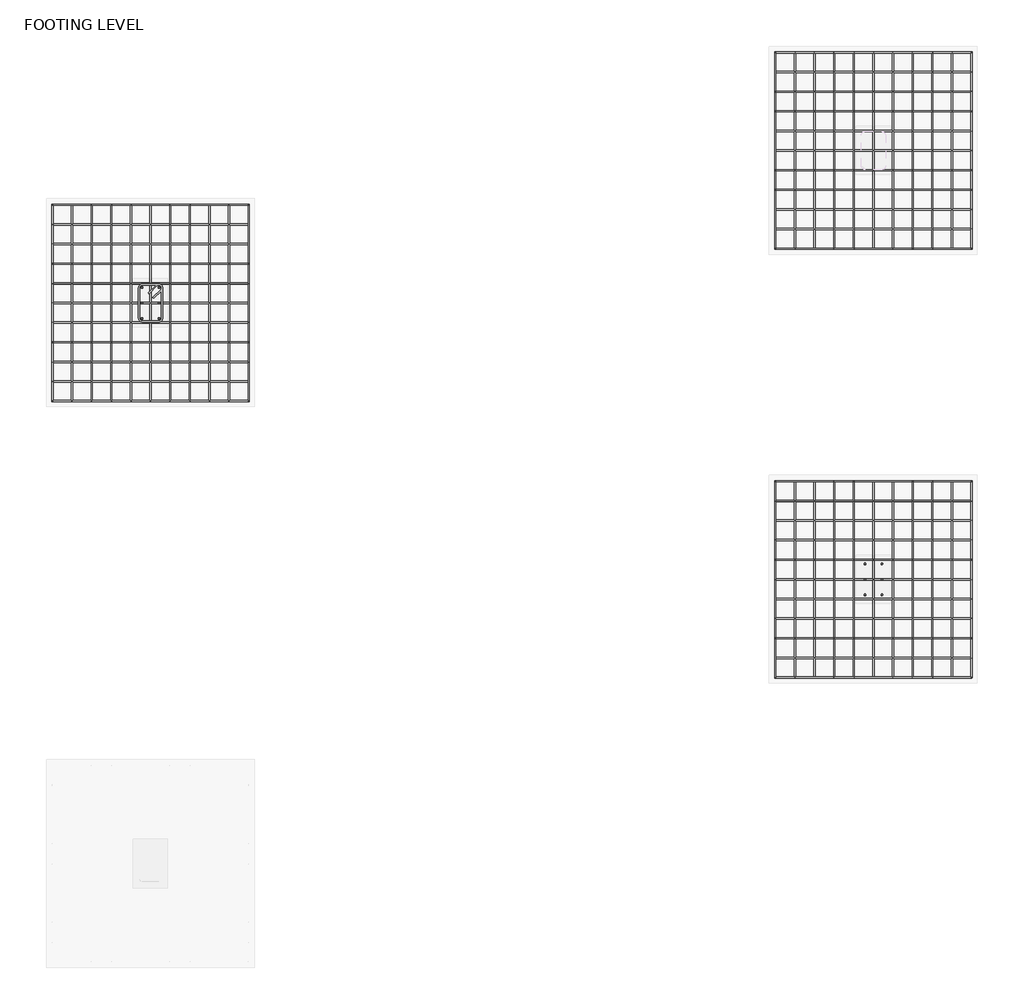
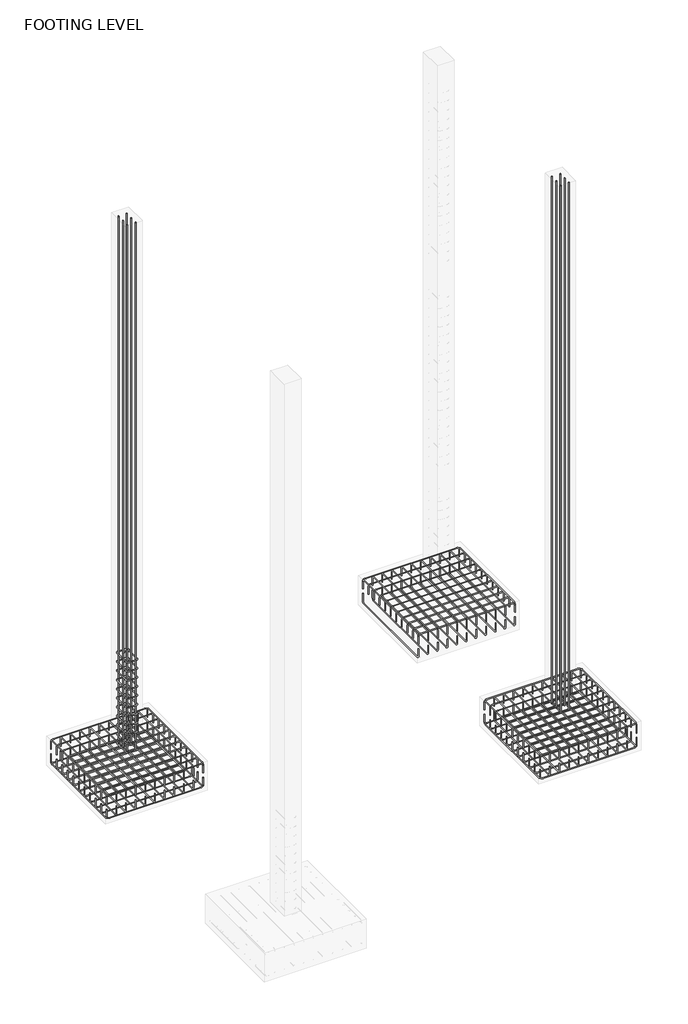
# One storey, part 5 of 9: 24 reinforcing bars.
"""IFC4 building model written with IfcOpenShell, lengths in millimetres."""

from ifc_helpers import new_model, si_unit, point, frame, origin, place, context, project, spatial, polyline, circle_curve, trimmed, segment, composite_curve, source, transform, mapped, element, save
from ifc_brep_helpers import swept_disk

model = new_model("IFC4")

# Units and contexts
model_context = context("Model", 3, world=origin())
ifc_project = project(units=[si_unit("LENGTHUNIT", "METRE", prefix="MILLI")], contexts=[model_context])

# Site, building, storey
site = spatial("IfcSite", under=ifc_project)
building = spatial("IfcBuilding", under=site)
storey = spatial("IfcBuildingStorey", under=building, Name="FOOTING LEVEL", Elevation=-1981.2)

# Reinforcing bars
placement = place(None, origin())
reinforcing_bar_shape = source(origin(), model_context, "Body", "SolidModel", [
    swept_disk(composite_curve([segment(polyline([(-2537.1816189, 2241.6973175, -2171.7), (-2537.1816189, 2241.6973175, -2057.4)]), True, "CONTINUOUS"), segment(trimmed(circle_curve(frame((-2537.1816189, 2208.3598175, -2057.4), z_axis=(1.0, 0.0, 0.0), x_axis=(0.0, 33.337499999999636, 0.0)), 33.3375), [point((-2537.1816189, 2241.6973175, -2057.4))], [point((-2537.1816189, 2208.3598175, -2024.0625))], True, "CARTESIAN"), True, "CONTINUOUS"), segment(polyline([(-2537.1816189, 2208.3598175, -2024.0625), (-2537.1816189, 836.7598175, -2024.0625)]), True, "CONTINUOUS"), segment(trimmed(circle_curve(frame((-2537.1816189, 836.7598175, -2057.4), z_axis=(1.0, 0.0, 0.0), x_axis=(0.0, 0.0, 33.33750000000009)), 33.3375), [point((-2537.1816189, 836.7598175, -2024.0625))], [point((-2537.1816189, 803.4223175, -2057.4))], True, "CARTESIAN"), True, "CONTINUOUS"), segment(polyline([(-2537.1816189, 803.4223175, -2057.4), (-2537.1816189, 803.4223175, -2171.7)]), True, "CONTINUOUS")], self_intersect=False), 4.7625),
])
element("IfcReinforcingBar", 1, at=placement, inside=storey, context=model_context, shape_type="MappedRepresentation", body=[
    mapped(reinforcing_bar_shape, transform((0.0, 0.0, 0.0), x_axis=(1.0, 0.0, 0.0), y_axis=(0.0, 1.0, 0.0), z_axis=(0.0, 0.0, 1.0))),
    mapped(reinforcing_bar_shape, transform((-143.8275, 0.0, 0.0), x_axis=(1.0, 0.0, 0.0), y_axis=(0.0, 1.0, 0.0), z_axis=(0.0, 0.0, 1.0))),
    mapped(reinforcing_bar_shape, transform((-287.655, 0.0, 0.0), x_axis=(1.0, 0.0, 0.0), y_axis=(0.0, 1.0, 0.0), z_axis=(0.0, 0.0, 1.0))),
    mapped(reinforcing_bar_shape, transform((-431.4825, 0.0, 0.0), x_axis=(1.0, 0.0, 0.0), y_axis=(0.0, 1.0, 0.0), z_axis=(0.0, 0.0, 1.0))),
    mapped(reinforcing_bar_shape, transform((-575.31, 0.0, 0.0), x_axis=(1.0, 0.0, 0.0), y_axis=(0.0, 1.0, 0.0), z_axis=(0.0, 0.0, 1.0))),
    mapped(reinforcing_bar_shape, transform((-719.1375, 0.0, 0.0), x_axis=(1.0, 0.0, 0.0), y_axis=(0.0, 1.0, 0.0), z_axis=(0.0, 0.0, 1.0))),
    mapped(reinforcing_bar_shape, transform((-862.965, 0.0, 0.0), x_axis=(1.0, 0.0, 0.0), y_axis=(0.0, 1.0, 0.0), z_axis=(0.0, 0.0, 1.0))),
    mapped(reinforcing_bar_shape, transform((-1006.7925, 0.0, 0.0), x_axis=(1.0, 0.0, 0.0), y_axis=(0.0, 1.0, 0.0), z_axis=(0.0, 0.0, 1.0))),
    mapped(reinforcing_bar_shape, transform((-1150.62, 0.0, 0.0), x_axis=(1.0, 0.0, 0.0), y_axis=(0.0, 1.0, 0.0), z_axis=(0.0, 0.0, 1.0))),
    mapped(reinforcing_bar_shape, transform((-1294.4475, 0.0, 0.0), x_axis=(1.0, 0.0, 0.0), y_axis=(0.0, 1.0, 0.0), z_axis=(0.0, 0.0, 1.0))),
    mapped(reinforcing_bar_shape, transform((-1438.275, 0.0, 0.0), x_axis=(1.0, 0.0, 0.0), y_axis=(0.0, 1.0, 0.0), z_axis=(0.0, 0.0, 1.0))),
])
reinforcing_bar_2_shape = source(origin(), model_context, "Body", "SolidModel", [
    swept_disk(composite_curve([segment(polyline([(-2537.1816189, 803.4223175, -2247.9), (-2537.1816189, 803.4223175, -2362.2)]), True, "CONTINUOUS"), segment(trimmed(circle_curve(frame((-2537.1816189, 836.7598175, -2362.2), z_axis=(1.0, 0.0, 0.0), x_axis=(0.0, -33.33750000000009, 0.0)), 33.3375), [point((-2537.1816189, 803.4223175, -2362.2))], [point((-2537.1816189, 836.7598175, -2395.5375))], True, "CARTESIAN"), True, "CONTINUOUS"), segment(polyline([(-2537.1816189, 836.7598175, -2395.5375), (-2537.1816189, 2208.3598175, -2395.5375)]), True, "CONTINUOUS"), segment(trimmed(circle_curve(frame((-2537.1816189, 2208.3598175, -2362.2), z_axis=(1.0, 0.0, 0.0), x_axis=(0.0, 0.0, -33.33750000000009)), 33.3375), [point((-2537.1816189, 2208.3598175, -2395.5375))], [point((-2537.1816189, 2241.6973175, -2362.2))], True, "CARTESIAN"), True, "CONTINUOUS"), segment(polyline([(-2537.1816189, 2241.6973175, -2362.2), (-2537.1816189, 2241.6973175, -2247.9)]), True, "CONTINUOUS")], self_intersect=False), 4.7625),
])
element("IfcReinforcingBar", 2, at=placement, inside=storey, context=model_context, shape_type="MappedRepresentation", body=[
    mapped(reinforcing_bar_2_shape, transform((0.0, 0.0, 0.0), x_axis=(1.0, 0.0, 0.0), y_axis=(0.0, 1.0, 0.0), z_axis=(0.0, 0.0, 1.0))),
    mapped(reinforcing_bar_2_shape, transform((-143.8275, 0.0, 0.0), x_axis=(1.0, 0.0, 0.0), y_axis=(0.0, 1.0, 0.0), z_axis=(0.0, 0.0, 1.0))),
    mapped(reinforcing_bar_2_shape, transform((-287.655, 0.0, 0.0), x_axis=(1.0, 0.0, 0.0), y_axis=(0.0, 1.0, 0.0), z_axis=(0.0, 0.0, 1.0))),
    mapped(reinforcing_bar_2_shape, transform((-431.4825, 0.0, 0.0), x_axis=(1.0, 0.0, 0.0), y_axis=(0.0, 1.0, 0.0), z_axis=(0.0, 0.0, 1.0))),
    mapped(reinforcing_bar_2_shape, transform((-575.31, 0.0, 0.0), x_axis=(1.0, 0.0, 0.0), y_axis=(0.0, 1.0, 0.0), z_axis=(0.0, 0.0, 1.0))),
    mapped(reinforcing_bar_2_shape, transform((-719.1375, 0.0, 0.0), x_axis=(1.0, 0.0, 0.0), y_axis=(0.0, 1.0, 0.0), z_axis=(0.0, 0.0, 1.0))),
    mapped(reinforcing_bar_2_shape, transform((-862.965, 0.0, 0.0), x_axis=(1.0, 0.0, 0.0), y_axis=(0.0, 1.0, 0.0), z_axis=(0.0, 0.0, 1.0))),
    mapped(reinforcing_bar_2_shape, transform((-1006.7925, 0.0, 0.0), x_axis=(1.0, 0.0, 0.0), y_axis=(0.0, 1.0, 0.0), z_axis=(0.0, 0.0, 1.0))),
    mapped(reinforcing_bar_2_shape, transform((-1150.62, 0.0, 0.0), x_axis=(1.0, 0.0, 0.0), y_axis=(0.0, 1.0, 0.0), z_axis=(0.0, 0.0, 1.0))),
    mapped(reinforcing_bar_2_shape, transform((-1294.4475, 0.0, 0.0), x_axis=(1.0, 0.0, 0.0), y_axis=(0.0, 1.0, 0.0), z_axis=(0.0, 0.0, 1.0))),
    mapped(reinforcing_bar_2_shape, transform((-1438.275, 0.0, 0.0), x_axis=(1.0, 0.0, 0.0), y_axis=(0.0, 1.0, 0.0), z_axis=(0.0, 0.0, 1.0))),
])
reinforcing_bar_3_shape = source(origin(), model_context, "Body", "SolidModel", [
    swept_disk(composite_curve([segment(polyline([(-3975.4566189, 2241.6973175, -2171.7), (-3975.4566189, 2241.6973175, -2057.4)]), True, "CONTINUOUS"), segment(trimmed(circle_curve(frame((-3942.1191189, 2241.6973175, -2057.4), z_axis=(0.0, 1.0, 0.0), x_axis=(-33.33750000000009, 0.0, 0.0)), 33.3375), [point((-3975.4566189, 2241.6973175, -2057.4))], [point((-3942.1191189, 2241.6973175, -2024.0625))], True, "CARTESIAN"), True, "CONTINUOUS"), segment(polyline([(-3942.1191189, 2241.6973175, -2024.0625), (-2570.5191189, 2241.6973175, -2024.0625)]), True, "CONTINUOUS"), segment(trimmed(circle_curve(frame((-2570.5191189, 2241.6973175, -2057.4), z_axis=(0.0, 1.0, 0.0), x_axis=(0.0, 0.0, 33.33750000000009)), 33.3375), [point((-2570.5191189, 2241.6973175, -2024.0625))], [point((-2537.1816189, 2241.6973175, -2057.4))], True, "CARTESIAN"), True, "CONTINUOUS"), segment(polyline([(-2537.1816189, 2241.6973175, -2057.4), (-2537.1816189, 2241.6973175, -2171.7)]), True, "CONTINUOUS")], self_intersect=False), 4.7625),
])
element("IfcReinforcingBar", 3, at=placement, inside=storey, context=model_context, shape_type="MappedRepresentation", body=[
    mapped(reinforcing_bar_3_shape, transform((0.0, 0.0, 0.0), x_axis=(1.0, 0.0, 0.0), y_axis=(0.0, 1.0, 0.0), z_axis=(0.0, 0.0, 1.0))),
    mapped(reinforcing_bar_3_shape, transform((0.0, -143.8275, 0.0), x_axis=(1.0, 0.0, 0.0), y_axis=(0.0, 1.0, 0.0), z_axis=(0.0, 0.0, 1.0))),
    mapped(reinforcing_bar_3_shape, transform((0.0, -287.655, 0.0), x_axis=(1.0, 0.0, 0.0), y_axis=(0.0, 1.0, 0.0), z_axis=(0.0, 0.0, 1.0))),
    mapped(reinforcing_bar_3_shape, transform((0.0, -431.4825, 0.0), x_axis=(1.0, 0.0, 0.0), y_axis=(0.0, 1.0, 0.0), z_axis=(0.0, 0.0, 1.0))),
    mapped(reinforcing_bar_3_shape, transform((0.0, -575.31, 0.0), x_axis=(1.0, 0.0, 0.0), y_axis=(0.0, 1.0, 0.0), z_axis=(0.0, 0.0, 1.0))),
    mapped(reinforcing_bar_3_shape, transform((0.0, -719.1375, 0.0), x_axis=(1.0, 0.0, 0.0), y_axis=(0.0, 1.0, 0.0), z_axis=(0.0, 0.0, 1.0))),
    mapped(reinforcing_bar_3_shape, transform((0.0, -862.965, 0.0), x_axis=(1.0, 0.0, 0.0), y_axis=(0.0, 1.0, 0.0), z_axis=(0.0, 0.0, 1.0))),
    mapped(reinforcing_bar_3_shape, transform((0.0, -1006.7925, 0.0), x_axis=(1.0, 0.0, 0.0), y_axis=(0.0, 1.0, 0.0), z_axis=(0.0, 0.0, 1.0))),
    mapped(reinforcing_bar_3_shape, transform((0.0, -1150.62, 0.0), x_axis=(1.0, 0.0, 0.0), y_axis=(0.0, 1.0, 0.0), z_axis=(0.0, 0.0, 1.0))),
    mapped(reinforcing_bar_3_shape, transform((0.0, -1294.4475, 0.0), x_axis=(1.0, 0.0, 0.0), y_axis=(0.0, 1.0, 0.0), z_axis=(0.0, 0.0, 1.0))),
    mapped(reinforcing_bar_3_shape, transform((0.0, -1438.275, 0.0), x_axis=(1.0, 0.0, 0.0), y_axis=(0.0, 1.0, 0.0), z_axis=(0.0, 0.0, 1.0))),
])
reinforcing_bar_4_shape = source(origin(), model_context, "Body", "SolidModel", [
    swept_disk(composite_curve([segment(polyline([(-3975.4566189, 803.4223175, -2247.9), (-3975.4566189, 803.4223175, -2362.2)]), True, "CONTINUOUS"), segment(trimmed(circle_curve(frame((-3942.1191189, 803.4223175, -2362.2), z_axis=(0.0, -1.0, 0.0), x_axis=(-33.33750000000009, 0.0, 0.0)), 33.3375), [point((-3975.4566189, 803.4223175, -2362.2))], [point((-3942.1191189, 803.4223175, -2395.5375))], True, "CARTESIAN"), True, "CONTINUOUS"), segment(polyline([(-3942.1191189, 803.4223175, -2395.5375), (-2570.5191189, 803.4223175, -2395.5375)]), True, "CONTINUOUS"), segment(trimmed(circle_curve(frame((-2570.5191189, 803.4223175, -2362.2), z_axis=(0.0, -1.0, 0.0), x_axis=(0.0, 0.0, -33.33750000000009)), 33.3375), [point((-2570.5191189, 803.4223175, -2395.5375))], [point((-2537.1816189, 803.4223175, -2362.2))], True, "CARTESIAN"), True, "CONTINUOUS"), segment(polyline([(-2537.1816189, 803.4223175, -2362.2), (-2537.1816189, 803.4223175, -2247.9)]), True, "CONTINUOUS")], self_intersect=False), 4.7625),
])
element("IfcReinforcingBar", 4, at=placement, inside=storey, context=model_context, shape_type="MappedRepresentation", body=[
    mapped(reinforcing_bar_4_shape, transform((0.0, 0.0, 0.0), x_axis=(1.0, 0.0, 0.0), y_axis=(0.0, 1.0, 0.0), z_axis=(0.0, 0.0, 1.0))),
    mapped(reinforcing_bar_4_shape, transform((0.0, 143.8275, 0.0), x_axis=(1.0, 0.0, 0.0), y_axis=(0.0, 1.0, 0.0), z_axis=(0.0, 0.0, 1.0))),
    mapped(reinforcing_bar_4_shape, transform((0.0, 287.655, 0.0), x_axis=(1.0, 0.0, 0.0), y_axis=(0.0, 1.0, 0.0), z_axis=(0.0, 0.0, 1.0))),
    mapped(reinforcing_bar_4_shape, transform((0.0, 431.4825, 0.0), x_axis=(1.0, 0.0, 0.0), y_axis=(0.0, 1.0, 0.0), z_axis=(0.0, 0.0, 1.0))),
    mapped(reinforcing_bar_4_shape, transform((0.0, 575.31, 0.0), x_axis=(1.0, 0.0, 0.0), y_axis=(0.0, 1.0, 0.0), z_axis=(0.0, 0.0, 1.0))),
    mapped(reinforcing_bar_4_shape, transform((0.0, 719.1375, 0.0), x_axis=(1.0, 0.0, 0.0), y_axis=(0.0, 1.0, 0.0), z_axis=(0.0, 0.0, 1.0))),
    mapped(reinforcing_bar_4_shape, transform((0.0, 862.965, 0.0), x_axis=(1.0, 0.0, 0.0), y_axis=(0.0, 1.0, 0.0), z_axis=(0.0, 0.0, 1.0))),
    mapped(reinforcing_bar_4_shape, transform((0.0, 1006.7925, 0.0), x_axis=(1.0, 0.0, 0.0), y_axis=(0.0, 1.0, 0.0), z_axis=(0.0, 0.0, 1.0))),
    mapped(reinforcing_bar_4_shape, transform((0.0, 1150.62, 0.0), x_axis=(1.0, 0.0, 0.0), y_axis=(0.0, 1.0, 0.0), z_axis=(0.0, 0.0, 1.0))),
    mapped(reinforcing_bar_4_shape, transform((0.0, 1294.4475, 0.0), x_axis=(1.0, 0.0, 0.0), y_axis=(0.0, 1.0, 0.0), z_axis=(0.0, 0.0, 1.0))),
    mapped(reinforcing_bar_4_shape, transform((0.0, 1438.275, 0.0), x_axis=(1.0, 0.0, 0.0), y_axis=(0.0, 1.0, 0.0), z_axis=(0.0, 0.0, 1.0))),
])
reinforcing_bar_5_shape = source(origin(), model_context, "Body", "SolidModel", [
    swept_disk(composite_curve([segment(polyline([(-2537.1816189, 5383.1869441, -2171.7), (-2537.1816189, 5383.1869441, -2057.4)]), True, "CONTINUOUS"), segment(trimmed(circle_curve(frame((-2537.1816189, 5349.8494441, -2057.4), z_axis=(1.0, 0.0, 0.0), x_axis=(0.0, 33.337499999999636, 0.0)), 33.3375), [point((-2537.1816189, 5383.1869441, -2057.4))], [point((-2537.1816189, 5349.8494441, -2024.0625))], True, "CARTESIAN"), True, "CONTINUOUS"), segment(polyline([(-2537.1816189, 5349.8494441, -2024.0625), (-2537.1816189, 3978.2494441, -2024.0625)]), True, "CONTINUOUS"), segment(trimmed(circle_curve(frame((-2537.1816189, 3978.2494441, -2057.4), z_axis=(1.0, 0.0, 0.0), x_axis=(0.0, 0.0, 33.33750000000009)), 33.3375), [point((-2537.1816189, 3978.2494441, -2024.0625))], [point((-2537.1816189, 3944.9119441, -2057.4))], True, "CARTESIAN"), True, "CONTINUOUS"), segment(polyline([(-2537.1816189, 3944.9119441, -2057.4), (-2537.1816189, 3944.9119441, -2171.7)]), True, "CONTINUOUS")], self_intersect=False), 4.7625),
])
element("IfcReinforcingBar", 5, at=placement, inside=storey, context=model_context, shape_type="MappedRepresentation", body=[
    mapped(reinforcing_bar_5_shape, transform((0.0, 0.0, 0.0), x_axis=(1.0, 0.0, 0.0), y_axis=(0.0, 1.0, 0.0), z_axis=(0.0, 0.0, 1.0))),
    mapped(reinforcing_bar_5_shape, transform((-143.8275, 0.0, 0.0), x_axis=(1.0, 0.0, 0.0), y_axis=(0.0, 1.0, 0.0), z_axis=(0.0, 0.0, 1.0))),
    mapped(reinforcing_bar_5_shape, transform((-287.655, 0.0, 0.0), x_axis=(1.0, 0.0, 0.0), y_axis=(0.0, 1.0, 0.0), z_axis=(0.0, 0.0, 1.0))),
    mapped(reinforcing_bar_5_shape, transform((-431.4825, 0.0, 0.0), x_axis=(1.0, 0.0, 0.0), y_axis=(0.0, 1.0, 0.0), z_axis=(0.0, 0.0, 1.0))),
    mapped(reinforcing_bar_5_shape, transform((-575.31, 0.0, 0.0), x_axis=(1.0, 0.0, 0.0), y_axis=(0.0, 1.0, 0.0), z_axis=(0.0, 0.0, 1.0))),
    mapped(reinforcing_bar_5_shape, transform((-719.1375, 0.0, 0.0), x_axis=(1.0, 0.0, 0.0), y_axis=(0.0, 1.0, 0.0), z_axis=(0.0, 0.0, 1.0))),
    mapped(reinforcing_bar_5_shape, transform((-862.965, 0.0, 0.0), x_axis=(1.0, 0.0, 0.0), y_axis=(0.0, 1.0, 0.0), z_axis=(0.0, 0.0, 1.0))),
    mapped(reinforcing_bar_5_shape, transform((-1006.7925, 0.0, 0.0), x_axis=(1.0, 0.0, 0.0), y_axis=(0.0, 1.0, 0.0), z_axis=(0.0, 0.0, 1.0))),
    mapped(reinforcing_bar_5_shape, transform((-1150.62, 0.0, 0.0), x_axis=(1.0, 0.0, 0.0), y_axis=(0.0, 1.0, 0.0), z_axis=(0.0, 0.0, 1.0))),
    mapped(reinforcing_bar_5_shape, transform((-1294.4475, 0.0, 0.0), x_axis=(1.0, 0.0, 0.0), y_axis=(0.0, 1.0, 0.0), z_axis=(0.0, 0.0, 1.0))),
    mapped(reinforcing_bar_5_shape, transform((-1438.275, 0.0, 0.0), x_axis=(1.0, 0.0, 0.0), y_axis=(0.0, 1.0, 0.0), z_axis=(0.0, 0.0, 1.0))),
])
reinforcing_bar_6_shape = source(origin(), model_context, "Body", "SolidModel", [
    swept_disk(composite_curve([segment(polyline([(-2537.1816189, 3944.9119441, -2247.9), (-2537.1816189, 3944.9119441, -2362.2)]), True, "CONTINUOUS"), segment(trimmed(circle_curve(frame((-2537.1816189, 3978.2494441, -2362.2), z_axis=(1.0, 0.0, 0.0), x_axis=(0.0, -33.33750000000009, 0.0)), 33.3375), [point((-2537.1816189, 3944.9119441, -2362.2))], [point((-2537.1816189, 3978.2494441, -2395.5375))], True, "CARTESIAN"), True, "CONTINUOUS"), segment(polyline([(-2537.1816189, 3978.2494441, -2395.5375), (-2537.1816189, 5349.8494441, -2395.5375)]), True, "CONTINUOUS"), segment(trimmed(circle_curve(frame((-2537.1816189, 5349.8494441, -2362.2), z_axis=(1.0, 0.0, 0.0), x_axis=(0.0, 0.0, -33.33750000000009)), 33.3375), [point((-2537.1816189, 5349.8494441, -2395.5375))], [point((-2537.1816189, 5383.1869441, -2362.2))], True, "CARTESIAN"), True, "CONTINUOUS"), segment(polyline([(-2537.1816189, 5383.1869441, -2362.2), (-2537.1816189, 5383.1869441, -2247.9)]), True, "CONTINUOUS")], self_intersect=False), 4.7625),
])
element("IfcReinforcingBar", 6, at=placement, inside=storey, context=model_context, shape_type="MappedRepresentation", body=[
    mapped(reinforcing_bar_6_shape, transform((0.0, 0.0, 0.0), x_axis=(1.0, 0.0, 0.0), y_axis=(0.0, 1.0, 0.0), z_axis=(0.0, 0.0, 1.0))),
    mapped(reinforcing_bar_6_shape, transform((-143.8275, 0.0, 0.0), x_axis=(1.0, 0.0, 0.0), y_axis=(0.0, 1.0, 0.0), z_axis=(0.0, 0.0, 1.0))),
    mapped(reinforcing_bar_6_shape, transform((-287.655, 0.0, 0.0), x_axis=(1.0, 0.0, 0.0), y_axis=(0.0, 1.0, 0.0), z_axis=(0.0, 0.0, 1.0))),
    mapped(reinforcing_bar_6_shape, transform((-431.4825, 0.0, 0.0), x_axis=(1.0, 0.0, 0.0), y_axis=(0.0, 1.0, 0.0), z_axis=(0.0, 0.0, 1.0))),
    mapped(reinforcing_bar_6_shape, transform((-575.31, 0.0, 0.0), x_axis=(1.0, 0.0, 0.0), y_axis=(0.0, 1.0, 0.0), z_axis=(0.0, 0.0, 1.0))),
    mapped(reinforcing_bar_6_shape, transform((-719.1375, 0.0, 0.0), x_axis=(1.0, 0.0, 0.0), y_axis=(0.0, 1.0, 0.0), z_axis=(0.0, 0.0, 1.0))),
    mapped(reinforcing_bar_6_shape, transform((-862.965, 0.0, 0.0), x_axis=(1.0, 0.0, 0.0), y_axis=(0.0, 1.0, 0.0), z_axis=(0.0, 0.0, 1.0))),
    mapped(reinforcing_bar_6_shape, transform((-1006.7925, 0.0, 0.0), x_axis=(1.0, 0.0, 0.0), y_axis=(0.0, 1.0, 0.0), z_axis=(0.0, 0.0, 1.0))),
    mapped(reinforcing_bar_6_shape, transform((-1150.62, 0.0, 0.0), x_axis=(1.0, 0.0, 0.0), y_axis=(0.0, 1.0, 0.0), z_axis=(0.0, 0.0, 1.0))),
    mapped(reinforcing_bar_6_shape, transform((-1294.4475, 0.0, 0.0), x_axis=(1.0, 0.0, 0.0), y_axis=(0.0, 1.0, 0.0), z_axis=(0.0, 0.0, 1.0))),
    mapped(reinforcing_bar_6_shape, transform((-1438.275, 0.0, 0.0), x_axis=(1.0, 0.0, 0.0), y_axis=(0.0, 1.0, 0.0), z_axis=(0.0, 0.0, 1.0))),
])
reinforcing_bar_7_shape = source(origin(), model_context, "Body", "SolidModel", [
    swept_disk(composite_curve([segment(polyline([(-3975.4566189, 5383.1869441, -2171.7), (-3975.4566189, 5383.1869441, -2057.4)]), True, "CONTINUOUS"), segment(trimmed(circle_curve(frame((-3942.1191189, 5383.1869441, -2057.4), z_axis=(0.0, 1.0, 0.0), x_axis=(-33.33750000000009, 0.0, 0.0)), 33.3375), [point((-3975.4566189, 5383.1869441, -2057.4))], [point((-3942.1191189, 5383.1869441, -2024.0625))], True, "CARTESIAN"), True, "CONTINUOUS"), segment(polyline([(-3942.1191189, 5383.1869441, -2024.0625), (-2570.5191189, 5383.1869441, -2024.0625)]), True, "CONTINUOUS"), segment(trimmed(circle_curve(frame((-2570.5191189, 5383.1869441, -2057.4), z_axis=(0.0, 1.0, 0.0), x_axis=(0.0, 0.0, 33.33750000000009)), 33.3375), [point((-2570.5191189, 5383.1869441, -2024.0625))], [point((-2537.1816189, 5383.1869441, -2057.4))], True, "CARTESIAN"), True, "CONTINUOUS"), segment(polyline([(-2537.1816189, 5383.1869441, -2057.4), (-2537.1816189, 5383.1869441, -2171.7)]), True, "CONTINUOUS")], self_intersect=False), 4.7625),
])
element("IfcReinforcingBar", 7, at=placement, inside=storey, context=model_context, shape_type="MappedRepresentation", body=[
    mapped(reinforcing_bar_7_shape, transform((0.0, 0.0, 0.0), x_axis=(1.0, 0.0, 0.0), y_axis=(0.0, 1.0, 0.0), z_axis=(0.0, 0.0, 1.0))),
    mapped(reinforcing_bar_7_shape, transform((0.0, -143.8275, 0.0), x_axis=(1.0, 0.0, 0.0), y_axis=(0.0, 1.0, 0.0), z_axis=(0.0, 0.0, 1.0))),
    mapped(reinforcing_bar_7_shape, transform((0.0, -287.655, 0.0), x_axis=(1.0, 0.0, 0.0), y_axis=(0.0, 1.0, 0.0), z_axis=(0.0, 0.0, 1.0))),
    mapped(reinforcing_bar_7_shape, transform((0.0, -431.4825, 0.0), x_axis=(1.0, 0.0, 0.0), y_axis=(0.0, 1.0, 0.0), z_axis=(0.0, 0.0, 1.0))),
    mapped(reinforcing_bar_7_shape, transform((0.0, -575.31, 0.0), x_axis=(1.0, 0.0, 0.0), y_axis=(0.0, 1.0, 0.0), z_axis=(0.0, 0.0, 1.0))),
    mapped(reinforcing_bar_7_shape, transform((0.0, -719.1375, 0.0), x_axis=(1.0, 0.0, 0.0), y_axis=(0.0, 1.0, 0.0), z_axis=(0.0, 0.0, 1.0))),
    mapped(reinforcing_bar_7_shape, transform((0.0, -862.965, 0.0), x_axis=(1.0, 0.0, 0.0), y_axis=(0.0, 1.0, 0.0), z_axis=(0.0, 0.0, 1.0))),
    mapped(reinforcing_bar_7_shape, transform((0.0, -1006.7925, 0.0), x_axis=(1.0, 0.0, 0.0), y_axis=(0.0, 1.0, 0.0), z_axis=(0.0, 0.0, 1.0))),
    mapped(reinforcing_bar_7_shape, transform((0.0, -1150.62, 0.0), x_axis=(1.0, 0.0, 0.0), y_axis=(0.0, 1.0, 0.0), z_axis=(0.0, 0.0, 1.0))),
    mapped(reinforcing_bar_7_shape, transform((0.0, -1294.4475, 0.0), x_axis=(1.0, 0.0, 0.0), y_axis=(0.0, 1.0, 0.0), z_axis=(0.0, 0.0, 1.0))),
    mapped(reinforcing_bar_7_shape, transform((0.0, -1438.275, 0.0), x_axis=(1.0, 0.0, 0.0), y_axis=(0.0, 1.0, 0.0), z_axis=(0.0, 0.0, 1.0))),
])
reinforcing_bar_8_shape = source(origin(), model_context, "Body", "SolidModel", [
    swept_disk(composite_curve([segment(polyline([(-7832.9458659, 4266.5658402, -2171.7), (-7832.9458659, 4266.5658402, -2057.4)]), True, "CONTINUOUS"), segment(trimmed(circle_curve(frame((-7832.9458659, 4233.2283402, -2057.4), z_axis=(1.0, 0.0, 0.0), x_axis=(0.0, 33.337499999999636, 0.0)), 33.3375), [point((-7832.9458659, 4266.5658402, -2057.4))], [point((-7832.9458659, 4233.2283402, -2024.0625))], True, "CARTESIAN"), True, "CONTINUOUS"), segment(polyline([(-7832.9458659, 4233.2283402, -2024.0625), (-7832.9458659, 2861.6283402, -2024.0625)]), True, "CONTINUOUS"), segment(trimmed(circle_curve(frame((-7832.9458659, 2861.6283402, -2057.4), z_axis=(1.0, 0.0, 0.0), x_axis=(0.0, 0.0, 33.33750000000009)), 33.3375), [point((-7832.9458659, 2861.6283402, -2024.0625))], [point((-7832.9458659, 2828.2908402, -2057.4))], True, "CARTESIAN"), True, "CONTINUOUS"), segment(polyline([(-7832.9458659, 2828.2908402, -2057.4), (-7832.9458659, 2828.2908402, -2171.7)]), True, "CONTINUOUS")], self_intersect=False), 4.7625),
])
element("IfcReinforcingBar", 8, at=placement, inside=storey, context=model_context, shape_type="MappedRepresentation", body=[
    mapped(reinforcing_bar_8_shape, transform((0.0, 0.0, 0.0), x_axis=(1.0, 0.0, 0.0), y_axis=(0.0, 1.0, 0.0), z_axis=(0.0, 0.0, 1.0))),
    mapped(reinforcing_bar_8_shape, transform((-143.8275, 0.0, 0.0), x_axis=(1.0, 0.0, 0.0), y_axis=(0.0, 1.0, 0.0), z_axis=(0.0, 0.0, 1.0))),
    mapped(reinforcing_bar_8_shape, transform((-287.655, 0.0, 0.0), x_axis=(1.0, 0.0, 0.0), y_axis=(0.0, 1.0, 0.0), z_axis=(0.0, 0.0, 1.0))),
    mapped(reinforcing_bar_8_shape, transform((-431.4825, 0.0, 0.0), x_axis=(1.0, 0.0, 0.0), y_axis=(0.0, 1.0, 0.0), z_axis=(0.0, 0.0, 1.0))),
    mapped(reinforcing_bar_8_shape, transform((-575.31, 0.0, 0.0), x_axis=(1.0, 0.0, 0.0), y_axis=(0.0, 1.0, 0.0), z_axis=(0.0, 0.0, 1.0))),
    mapped(reinforcing_bar_8_shape, transform((-719.1375, 0.0, 0.0), x_axis=(1.0, 0.0, 0.0), y_axis=(0.0, 1.0, 0.0), z_axis=(0.0, 0.0, 1.0))),
    mapped(reinforcing_bar_8_shape, transform((-862.965, 0.0, 0.0), x_axis=(1.0, 0.0, 0.0), y_axis=(0.0, 1.0, 0.0), z_axis=(0.0, 0.0, 1.0))),
    mapped(reinforcing_bar_8_shape, transform((-1006.7925, 0.0, 0.0), x_axis=(1.0, 0.0, 0.0), y_axis=(0.0, 1.0, 0.0), z_axis=(0.0, 0.0, 1.0))),
    mapped(reinforcing_bar_8_shape, transform((-1150.62, 0.0, 0.0), x_axis=(1.0, 0.0, 0.0), y_axis=(0.0, 1.0, 0.0), z_axis=(0.0, 0.0, 1.0))),
    mapped(reinforcing_bar_8_shape, transform((-1294.4475, 0.0, 0.0), x_axis=(1.0, 0.0, 0.0), y_axis=(0.0, 1.0, 0.0), z_axis=(0.0, 0.0, 1.0))),
    mapped(reinforcing_bar_8_shape, transform((-1438.275, 0.0, 0.0), x_axis=(1.0, 0.0, 0.0), y_axis=(0.0, 1.0, 0.0), z_axis=(0.0, 0.0, 1.0))),
])
reinforcing_bar_9_shape = source(origin(), model_context, "Body", "SolidModel", [
    swept_disk(composite_curve([segment(polyline([(-7832.9458659, 2828.2908402, -2247.9), (-7832.9458659, 2828.2908402, -2362.2)]), True, "CONTINUOUS"), segment(trimmed(circle_curve(frame((-7832.9458659, 2861.6283402, -2362.2), z_axis=(1.0, 0.0, 0.0), x_axis=(0.0, -33.33750000000009, 0.0)), 33.3375), [point((-7832.9458659, 2828.2908402, -2362.2))], [point((-7832.9458659, 2861.6283402, -2395.5375))], True, "CARTESIAN"), True, "CONTINUOUS"), segment(polyline([(-7832.9458659, 2861.6283402, -2395.5375), (-7832.9458659, 4233.2283402, -2395.5375)]), True, "CONTINUOUS"), segment(trimmed(circle_curve(frame((-7832.9458659, 4233.2283402, -2362.2), z_axis=(1.0, 0.0, 0.0), x_axis=(0.0, 0.0, -33.33750000000009)), 33.3375), [point((-7832.9458659, 4233.2283402, -2395.5375))], [point((-7832.9458659, 4266.5658402, -2362.2))], True, "CARTESIAN"), True, "CONTINUOUS"), segment(polyline([(-7832.9458659, 4266.5658402, -2362.2), (-7832.9458659, 4266.5658402, -2247.9)]), True, "CONTINUOUS")], self_intersect=False), 4.7625),
])
element("IfcReinforcingBar", 9, at=placement, inside=storey, context=model_context, shape_type="MappedRepresentation", body=[
    mapped(reinforcing_bar_9_shape, transform((0.0, 0.0, 0.0), x_axis=(1.0, 0.0, 0.0), y_axis=(0.0, 1.0, 0.0), z_axis=(0.0, 0.0, 1.0))),
    mapped(reinforcing_bar_9_shape, transform((-143.8275, 0.0, 0.0), x_axis=(1.0, 0.0, 0.0), y_axis=(0.0, 1.0, 0.0), z_axis=(0.0, 0.0, 1.0))),
    mapped(reinforcing_bar_9_shape, transform((-287.655, 0.0, 0.0), x_axis=(1.0, 0.0, 0.0), y_axis=(0.0, 1.0, 0.0), z_axis=(0.0, 0.0, 1.0))),
    mapped(reinforcing_bar_9_shape, transform((-431.4825, 0.0, 0.0), x_axis=(1.0, 0.0, 0.0), y_axis=(0.0, 1.0, 0.0), z_axis=(0.0, 0.0, 1.0))),
    mapped(reinforcing_bar_9_shape, transform((-575.31, 0.0, 0.0), x_axis=(1.0, 0.0, 0.0), y_axis=(0.0, 1.0, 0.0), z_axis=(0.0, 0.0, 1.0))),
    mapped(reinforcing_bar_9_shape, transform((-719.1375, 0.0, 0.0), x_axis=(1.0, 0.0, 0.0), y_axis=(0.0, 1.0, 0.0), z_axis=(0.0, 0.0, 1.0))),
    mapped(reinforcing_bar_9_shape, transform((-862.965, 0.0, 0.0), x_axis=(1.0, 0.0, 0.0), y_axis=(0.0, 1.0, 0.0), z_axis=(0.0, 0.0, 1.0))),
    mapped(reinforcing_bar_9_shape, transform((-1006.7925, 0.0, 0.0), x_axis=(1.0, 0.0, 0.0), y_axis=(0.0, 1.0, 0.0), z_axis=(0.0, 0.0, 1.0))),
    mapped(reinforcing_bar_9_shape, transform((-1150.62, 0.0, 0.0), x_axis=(1.0, 0.0, 0.0), y_axis=(0.0, 1.0, 0.0), z_axis=(0.0, 0.0, 1.0))),
    mapped(reinforcing_bar_9_shape, transform((-1294.4475, 0.0, 0.0), x_axis=(1.0, 0.0, 0.0), y_axis=(0.0, 1.0, 0.0), z_axis=(0.0, 0.0, 1.0))),
    mapped(reinforcing_bar_9_shape, transform((-1438.275, 0.0, 0.0), x_axis=(1.0, 0.0, 0.0), y_axis=(0.0, 1.0, 0.0), z_axis=(0.0, 0.0, 1.0))),
])
reinforcing_bar_10_shape = source(origin(), model_context, "Body", "SolidModel", [
    swept_disk(composite_curve([segment(polyline([(-9271.2208659, 4266.5658402, -2171.7), (-9271.2208659, 4266.5658402, -2057.4)]), True, "CONTINUOUS"), segment(trimmed(circle_curve(frame((-9237.8833659, 4266.5658402, -2057.4), z_axis=(0.0, 1.0, 0.0), x_axis=(-33.337500000001455, 0.0, 0.0)), 33.3375), [point((-9271.2208659, 4266.5658402, -2057.4))], [point((-9237.8833659, 4266.5658402, -2024.0625))], True, "CARTESIAN"), True, "CONTINUOUS"), segment(polyline([(-9237.8833659, 4266.5658402, -2024.0625), (-7866.2833659, 4266.5658402, -2024.0625)]), True, "CONTINUOUS"), segment(trimmed(circle_curve(frame((-7866.2833659, 4266.5658402, -2057.4), z_axis=(0.0, 1.0, 0.0), x_axis=(0.0, 0.0, 33.33750000000009)), 33.3375), [point((-7866.2833659, 4266.5658402, -2024.0625))], [point((-7832.9458659, 4266.5658402, -2057.4))], True, "CARTESIAN"), True, "CONTINUOUS"), segment(polyline([(-7832.9458659, 4266.5658402, -2057.4), (-7832.9458659, 4266.5658402, -2171.7)]), True, "CONTINUOUS")], self_intersect=False), 4.7625),
])
element("IfcReinforcingBar", 10, at=placement, inside=storey, context=model_context, shape_type="MappedRepresentation", body=[
    mapped(reinforcing_bar_10_shape, transform((0.0, 0.0, 0.0), x_axis=(1.0, 0.0, 0.0), y_axis=(0.0, 1.0, 0.0), z_axis=(0.0, 0.0, 1.0))),
    mapped(reinforcing_bar_10_shape, transform((0.0, -143.8275, 0.0), x_axis=(1.0, 0.0, 0.0), y_axis=(0.0, 1.0, 0.0), z_axis=(0.0, 0.0, 1.0))),
    mapped(reinforcing_bar_10_shape, transform((0.0, -287.655, 0.0), x_axis=(1.0, 0.0, 0.0), y_axis=(0.0, 1.0, 0.0), z_axis=(0.0, 0.0, 1.0))),
    mapped(reinforcing_bar_10_shape, transform((0.0, -431.4825, 0.0), x_axis=(1.0, 0.0, 0.0), y_axis=(0.0, 1.0, 0.0), z_axis=(0.0, 0.0, 1.0))),
    mapped(reinforcing_bar_10_shape, transform((0.0, -575.31, 0.0), x_axis=(1.0, 0.0, 0.0), y_axis=(0.0, 1.0, 0.0), z_axis=(0.0, 0.0, 1.0))),
    mapped(reinforcing_bar_10_shape, transform((0.0, -719.1375, 0.0), x_axis=(1.0, 0.0, 0.0), y_axis=(0.0, 1.0, 0.0), z_axis=(0.0, 0.0, 1.0))),
    mapped(reinforcing_bar_10_shape, transform((0.0, -862.965, 0.0), x_axis=(1.0, 0.0, 0.0), y_axis=(0.0, 1.0, 0.0), z_axis=(0.0, 0.0, 1.0))),
    mapped(reinforcing_bar_10_shape, transform((0.0, -1006.7925, 0.0), x_axis=(1.0, 0.0, 0.0), y_axis=(0.0, 1.0, 0.0), z_axis=(0.0, 0.0, 1.0))),
    mapped(reinforcing_bar_10_shape, transform((0.0, -1150.62, 0.0), x_axis=(1.0, 0.0, 0.0), y_axis=(0.0, 1.0, 0.0), z_axis=(0.0, 0.0, 1.0))),
    mapped(reinforcing_bar_10_shape, transform((0.0, -1294.4475, 0.0), x_axis=(1.0, 0.0, 0.0), y_axis=(0.0, 1.0, 0.0), z_axis=(0.0, 0.0, 1.0))),
    mapped(reinforcing_bar_10_shape, transform((0.0, -1438.275, 0.0), x_axis=(1.0, 0.0, 0.0), y_axis=(0.0, 1.0, 0.0), z_axis=(0.0, 0.0, 1.0))),
])
reinforcing_bar_11_shape = source(origin(), model_context, "Body", "SolidModel", [
    swept_disk(composite_curve([segment(polyline([(-9271.2208659, 2828.2908402, -2247.9), (-9271.2208659, 2828.2908402, -2362.2)]), True, "CONTINUOUS"), segment(trimmed(circle_curve(frame((-9237.8833659, 2828.2908402, -2362.2), z_axis=(0.0, -1.0, 0.0), x_axis=(-33.337500000001455, 0.0, 0.0)), 33.3375), [point((-9271.2208659, 2828.2908402, -2362.2))], [point((-9237.8833659, 2828.2908402, -2395.5375))], True, "CARTESIAN"), True, "CONTINUOUS"), segment(polyline([(-9237.8833659, 2828.2908402, -2395.5375), (-7866.2833659, 2828.2908402, -2395.5375)]), True, "CONTINUOUS"), segment(trimmed(circle_curve(frame((-7866.2833659, 2828.2908402, -2362.2), z_axis=(0.0, -1.0, 0.0), x_axis=(0.0, 0.0, -33.33750000000009)), 33.3375), [point((-7866.2833659, 2828.2908402, -2395.5375))], [point((-7832.9458659, 2828.2908402, -2362.2))], True, "CARTESIAN"), True, "CONTINUOUS"), segment(polyline([(-7832.9458659, 2828.2908402, -2362.2), (-7832.9458659, 2828.2908402, -2247.9)]), True, "CONTINUOUS")], self_intersect=False), 4.7625),
])
element("IfcReinforcingBar", 11, at=placement, inside=storey, context=model_context, shape_type="MappedRepresentation", body=[
    mapped(reinforcing_bar_11_shape, transform((0.0, 0.0, 0.0), x_axis=(1.0, 0.0, 0.0), y_axis=(0.0, 1.0, 0.0), z_axis=(0.0, 0.0, 1.0))),
    mapped(reinforcing_bar_11_shape, transform((0.0, 143.8275, 0.0), x_axis=(1.0, 0.0, 0.0), y_axis=(0.0, 1.0, 0.0), z_axis=(0.0, 0.0, 1.0))),
    mapped(reinforcing_bar_11_shape, transform((0.0, 287.655, 0.0), x_axis=(1.0, 0.0, 0.0), y_axis=(0.0, 1.0, 0.0), z_axis=(0.0, 0.0, 1.0))),
    mapped(reinforcing_bar_11_shape, transform((0.0, 431.4825, 0.0), x_axis=(1.0, 0.0, 0.0), y_axis=(0.0, 1.0, 0.0), z_axis=(0.0, 0.0, 1.0))),
    mapped(reinforcing_bar_11_shape, transform((0.0, 575.31, 0.0), x_axis=(1.0, 0.0, 0.0), y_axis=(0.0, 1.0, 0.0), z_axis=(0.0, 0.0, 1.0))),
    mapped(reinforcing_bar_11_shape, transform((0.0, 719.1375, 0.0), x_axis=(1.0, 0.0, 0.0), y_axis=(0.0, 1.0, 0.0), z_axis=(0.0, 0.0, 1.0))),
    mapped(reinforcing_bar_11_shape, transform((0.0, 862.965, 0.0), x_axis=(1.0, 0.0, 0.0), y_axis=(0.0, 1.0, 0.0), z_axis=(0.0, 0.0, 1.0))),
    mapped(reinforcing_bar_11_shape, transform((0.0, 1006.7925, 0.0), x_axis=(1.0, 0.0, 0.0), y_axis=(0.0, 1.0, 0.0), z_axis=(0.0, 0.0, 1.0))),
    mapped(reinforcing_bar_11_shape, transform((0.0, 1150.62, 0.0), x_axis=(1.0, 0.0, 0.0), y_axis=(0.0, 1.0, 0.0), z_axis=(0.0, 0.0, 1.0))),
    mapped(reinforcing_bar_11_shape, transform((0.0, 1294.4475, 0.0), x_axis=(1.0, 0.0, 0.0), y_axis=(0.0, 1.0, 0.0), z_axis=(0.0, 0.0, 1.0))),
    mapped(reinforcing_bar_11_shape, transform((0.0, 1438.275, 0.0), x_axis=(1.0, 0.0, 0.0), y_axis=(0.0, 1.0, 0.0), z_axis=(0.0, 0.0, 1.0))),
])
reinforcing_bar_12_shape = source(origin(), model_context, "Body", "SolidModel", [
    swept_disk(composite_curve([segment(polyline([(-8531.7845827, 3584.8511629, -1938.3375), (-8474.9203857, 3641.71536, -1938.3375)]), True, "CONTINUOUS"), segment(trimmed(circle_curve(frame((-8491.7583659, 3658.5533402, -1938.3375), z_axis=(0.0, 0.0, 1.0), x_axis=(16.837980199999947, -16.837980199999947, 0.0)), 23.8125), [point((-8474.9203857, 3641.71536, -1938.3375))], [point((-8491.7583659, 3682.3658402, -1938.3375))], True, "CARTESIAN"), True, "CONTINUOUS"), segment(polyline([(-8491.7583659, 3682.3658402, -1938.3375), (-8612.4083659, 3682.3658402, -1938.3375)]), True, "CONTINUOUS"), segment(trimmed(circle_curve(frame((-8612.4083659, 3658.5533402, -1938.3375), z_axis=(0.0, 0.0, 1.0), x_axis=(0.0, 23.8125, 0.0)), 23.8125), [point((-8612.4083659, 3682.3658402, -1938.3375))], [point((-8636.2208659, 3658.5533402, -1938.3375))], True, "CARTESIAN"), True, "CONTINUOUS"), segment(polyline([(-8636.2208659, 3658.5533402, -1938.3375), (-8636.2208659, 3436.3033402, -1938.3375)]), True, "CONTINUOUS"), segment(trimmed(circle_curve(frame((-8612.4464219, 3436.3033402, -1939.6832232), z_axis=(0.056513312022656255, 0.0, 0.9984018457335854), x_axis=(-23.774444000000585, 0.0, 1.3457231999998385)), 23.8125), [point((-8636.2208659, 3436.3033402, -1938.3375))], [point((-8612.4464219, 3412.4908402, -1939.6832232))], True, "CARTESIAN"), True, "CONTINUOUS"), segment(polyline([(-8612.4464219, 3412.4908402, -1939.6832232), (-8491.7203098, 3412.4908402, -1946.5167768)]), True, "CONTINUOUS"), segment(trimmed(circle_curve(frame((-8491.7203098, 3436.3033402, -1946.5167768), z_axis=(0.056513312022656255, 0.0, 0.9984018457335854), x_axis=(0.0, -23.8125, 0.0)), 23.8125), [point((-8491.7203098, 3412.4908402, -1946.5167768))], [point((-8467.9458659, 3436.3033402, -1947.8625))], True, "CARTESIAN"), True, "CONTINUOUS"), segment(polyline([(-8467.9458659, 3436.3033402, -1947.8625), (-8467.9458659, 3658.5533402, -1947.8625)]), True, "CONTINUOUS"), segment(trimmed(circle_curve(frame((-8491.7583659, 3658.5533402, -1947.8625), z_axis=(0.0, 0.0, 1.0), x_axis=(23.8125, 0.0, 0.0)), 23.8125), [point((-8467.9458659, 3658.5533402, -1947.8625))], [point((-8508.5963461, 3675.3913204, -1947.8625))], True, "CARTESIAN"), True, "CONTINUOUS"), segment(polyline([(-8508.5963461, 3675.3913204, -1947.8625), (-8565.4605432, 3618.5271233, -1947.8625)]), True, "CONTINUOUS")], self_intersect=False), 4.7625),
])
element("IfcReinforcingBar", 12, at=placement, inside=storey, context=model_context, shape_type="MappedRepresentation", body=[
    mapped(reinforcing_bar_12_shape, transform((0.0, 0.0, 0.0), x_axis=(1.0, 0.0, 0.0), y_axis=(0.0, 1.0, 0.0), z_axis=(0.0, 0.0, 1.0))),
    mapped(reinforcing_bar_12_shape, transform((0.0, 0.0, 142.5866456), x_axis=(1.0, 0.0, 0.0), y_axis=(0.0, 1.0, 0.0), z_axis=(0.0, 0.0, 1.0))),
    mapped(reinforcing_bar_12_shape, transform((0.0, 0.0, 285.1732912), x_axis=(1.0, 0.0, 0.0), y_axis=(0.0, 1.0, 0.0), z_axis=(0.0, 0.0, 1.0))),
    mapped(reinforcing_bar_12_shape, transform((0.0, 0.0, 427.7599369), x_axis=(1.0, 0.0, 0.0), y_axis=(0.0, 1.0, 0.0), z_axis=(0.0, 0.0, 1.0))),
    mapped(reinforcing_bar_12_shape, transform((0.0, 0.0, 570.3465825), x_axis=(1.0, 0.0, 0.0), y_axis=(0.0, 1.0, 0.0), z_axis=(0.0, 0.0, 1.0))),
    mapped(reinforcing_bar_12_shape, transform((0.0, 0.0, 712.9332281), x_axis=(1.0, 0.0, 0.0), y_axis=(0.0, 1.0, 0.0), z_axis=(0.0, 0.0, 1.0))),
    mapped(reinforcing_bar_12_shape, transform((0.0, 0.0, 855.5198737), x_axis=(1.0, 0.0, 0.0), y_axis=(0.0, 1.0, 0.0), z_axis=(0.0, 0.0, 1.0))),
    mapped(reinforcing_bar_12_shape, transform((0.0, 0.0, 998.1065193), x_axis=(1.0, 0.0, 0.0), y_axis=(0.0, 1.0, 0.0), z_axis=(0.0, 0.0, 1.0))),
    mapped(reinforcing_bar_12_shape, transform((0.0, 0.0, 1140.6931649), x_axis=(1.0, 0.0, 0.0), y_axis=(0.0, 1.0, 0.0), z_axis=(0.0, 0.0, 1.0))),
    mapped(reinforcing_bar_12_shape, transform((0.0, 0.0, 1283.2798106), x_axis=(1.0, 0.0, 0.0), y_axis=(0.0, 1.0, 0.0), z_axis=(0.0, 0.0, 1.0))),
    mapped(reinforcing_bar_12_shape, transform((0.0, 0.0, 1425.8664562), x_axis=(1.0, 0.0, 0.0), y_axis=(0.0, 1.0, 0.0), z_axis=(0.0, 0.0, 1.0))),
])
element("IfcReinforcingBar", 13, at=placement, inside=storey, context=model_context, shape_type="SolidModel", body=[
    swept_disk(composite_curve([segment(polyline([(-8490.2784581, 3433.9470011, -1943.1), (-8490.2784581, 3433.9470011, 6362.7)]), True, "CONTINUOUS")], self_intersect=False), 6.35),
])
element("IfcReinforcingBar", 14, at=placement, inside=storey, context=model_context, shape_type="SolidModel", body=[
    swept_disk(composite_curve([segment(polyline([(-8613.8882737, 3433.9470011, -1943.1), (-8613.8882737, 3433.9470011, 6362.7)]), True, "CONTINUOUS")], self_intersect=False), 6.35),
])
element("IfcReinforcingBar", 15, at=placement, inside=storey, context=model_context, shape_type="SolidModel", body=[
    swept_disk(composite_curve([segment(polyline([(-8490.2784581, 3660.9096793, -1943.1), (-8490.2784581, 3660.9096793, 6362.7)]), True, "CONTINUOUS")], self_intersect=False), 6.35),
])
element("IfcReinforcingBar", 16, at=placement, inside=storey, context=model_context, shape_type="SolidModel", body=[
    swept_disk(composite_curve([segment(polyline([(-8613.8882737, 3660.9096793, -1943.1), (-8613.8882737, 3660.9096793, 6362.7)]), True, "CONTINUOUS")], self_intersect=False), 6.35),
])
element("IfcReinforcingBar", 17, at=placement, inside=storey, context=model_context, shape_type="SolidModel", body=[
    swept_disk(composite_curve([segment(polyline([(-8490.2784581, 3546.6096793, -1943.1), (-8490.2784581, 3546.6096793, 6362.7)]), True, "CONTINUOUS")], self_intersect=False), 6.35),
])
element("IfcReinforcingBar", 18, at=placement, inside=storey, context=model_context, shape_type="SolidModel", body=[
    swept_disk(composite_curve([segment(polyline([(-8613.8882737, 3546.6096793, -1943.1), (-8613.8882737, 3546.6096793, 6362.7)]), True, "CONTINUOUS")], self_intersect=False), 6.35),
])
element("IfcReinforcingBar", 19, at=placement, inside=storey, context=model_context, shape_type="SolidModel", body=[
    swept_disk(composite_curve([segment(polyline([(-3194.5142111, 1409.0784784, -1943.1), (-3194.5142111, 1409.0784784, 6362.7)]), True, "CONTINUOUS")], self_intersect=False), 6.35),
])
element("IfcReinforcingBar", 20, at=placement, inside=storey, context=model_context, shape_type="SolidModel", body=[
    swept_disk(composite_curve([segment(polyline([(-3318.1240267, 1409.0784784, -1943.1), (-3318.1240267, 1409.0784784, 6362.7)]), True, "CONTINUOUS")], self_intersect=False), 6.35),
])
element("IfcReinforcingBar", 21, at=placement, inside=storey, context=model_context, shape_type="SolidModel", body=[
    swept_disk(composite_curve([segment(polyline([(-3194.5142111, 1636.0411566, -1943.1), (-3194.5142111, 1636.0411566, 6362.7)]), True, "CONTINUOUS")], self_intersect=False), 6.35),
])
element("IfcReinforcingBar", 22, at=placement, inside=storey, context=model_context, shape_type="SolidModel", body=[
    swept_disk(composite_curve([segment(polyline([(-3318.1240267, 1636.0411566, -1943.1), (-3318.1240267, 1636.0411566, 6362.7)]), True, "CONTINUOUS")], self_intersect=False), 6.35),
])
element("IfcReinforcingBar", 23, at=placement, inside=storey, context=model_context, shape_type="SolidModel", body=[
    swept_disk(composite_curve([segment(polyline([(-3194.5142111, 1521.7411566, -1943.1), (-3194.5142111, 1521.7411566, 6362.7)]), True, "CONTINUOUS")], self_intersect=False), 6.35),
])
element("IfcReinforcingBar", 24, at=placement, inside=storey, context=model_context, shape_type="SolidModel", body=[
    swept_disk(composite_curve([segment(polyline([(-3318.1240267, 1521.7411566, -1943.1), (-3318.1240267, 1521.7411566, 6362.7)]), True, "CONTINUOUS")], self_intersect=False), 6.35),
])

save(model, "model.ifc")

# Revit data of these elements
# Elements 1, 2, 3, 4, 5, 6, 7, 8, 9, 10, 11, 12, 13, 14, 15, 16, 17, 18, 19, 20, 21, 22, 23, 24 (IfcReinforcingBar)
#   Phase Created = New Construction
